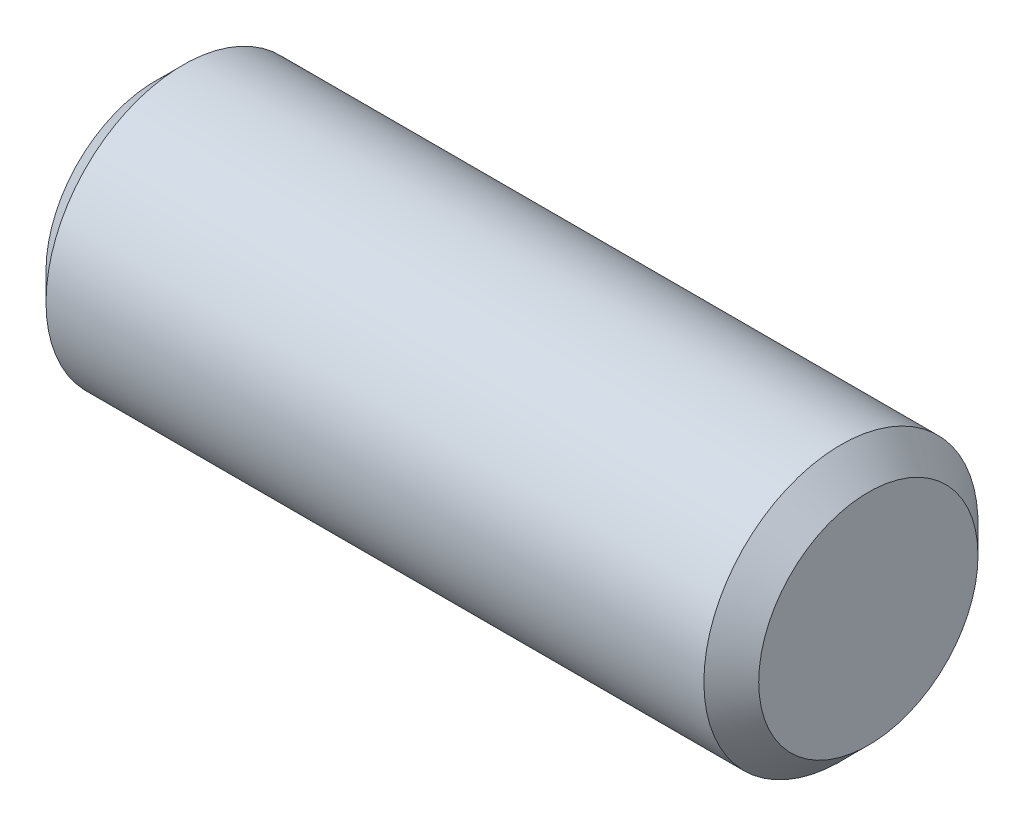
from build123d import *

# Parameters (mm, degrees)
PIN_PROFILE_20_R       = 10
PIN_BODY_20X52_DEPTH   = 26
END_CHAMFERS_2X45_SIZE = 2


with BuildPart() as part:
    # Pin Profile Ø20 → Pin Body Ø20x52 (new, symmetric)
    with BuildSketch(Plane(origin=(0, 0, 0), x_dir=(0, 0, -1), z_dir=(1, 0, 0))):
        with Locations(Location((0, 0, 0), (0, 0, 180))):
            Circle(PIN_PROFILE_20_R)
    extrude(amount=PIN_BODY_20X52_DEPTH, both=True)

    # End Chamfers 2x45°
    end_chamfers_2x45_edges = [part.edges().sort_by_distance(p)[0] for p in [
        (-26, 0, -10),
        (26, 0, -10),
    ]]
    chamfer(end_chamfers_2x45_edges, length=END_CHAMFERS_2X45_SIZE)


solid = part.part
